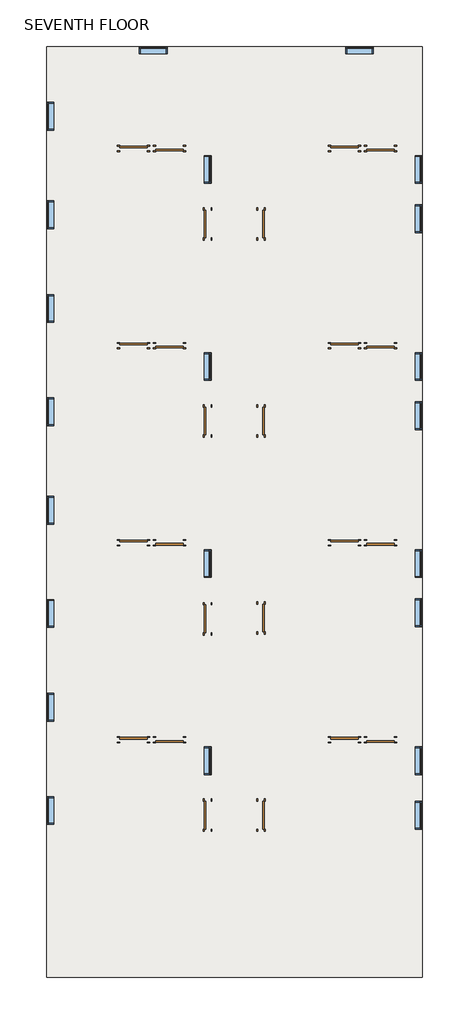
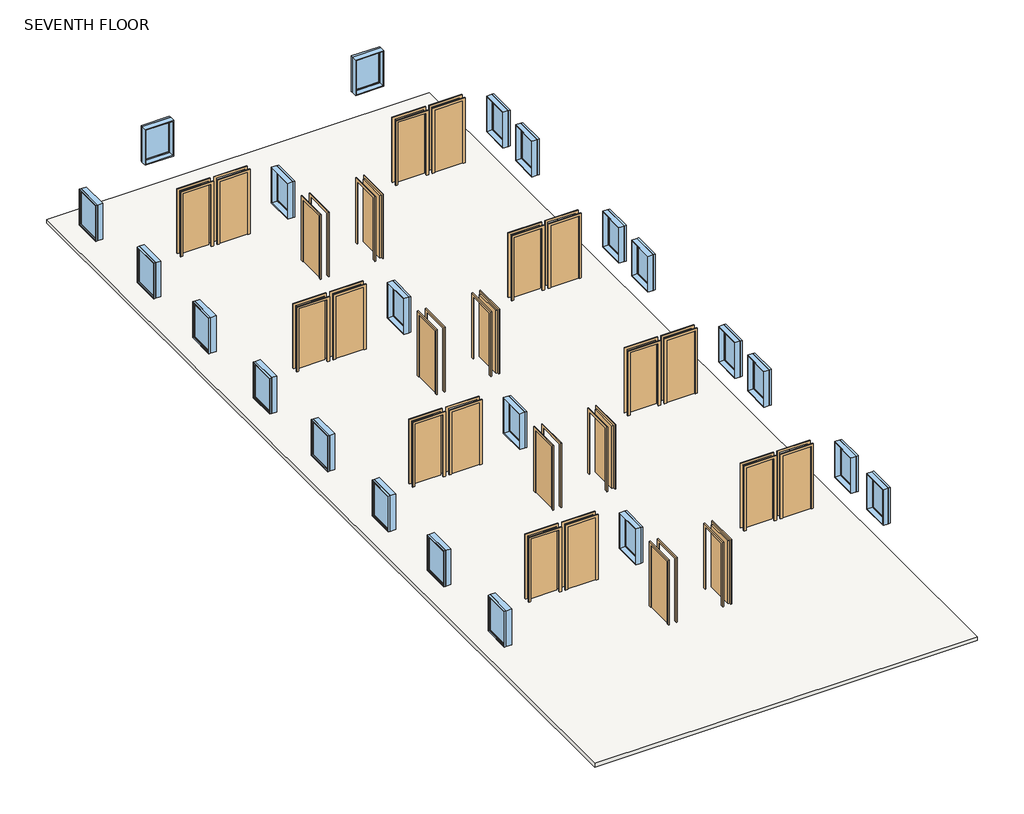
# One storey: 24 doors, 22 windows, 1 slab.
"""IFC4 building model written with IfcOpenShell, lengths in millimetres."""

from ifc_helpers import new_model, si_unit, frame, origin, place, context, project, spatial, polyline, outline, extrude, transform, mapped, element, save
from components import door_686f89d2, door_16372e1c, door_a90ba1ad, door_0ca8825f, window_c1f32544

model = new_model("IFC4")

# Units and contexts
model_context = context("Model", 3, world=origin())
ifc_project = project(units=[si_unit("LENGTHUNIT", "METRE", prefix="MILLI")], contexts=[model_context])

# Site, building, storey
site = spatial("IfcSite", under=ifc_project)
building = spatial("IfcBuilding", under=site)
storey = spatial("IfcBuildingStorey", under=building, Name="SEVENTH FLOOR", Elevation=22402.8)

# Doors
placement = place(None, origin())
door_shape = door_686f89d2(model_context)
element("IfcDoor", 1, ObjectType="Single-Flush : 36\" x 84\"", at=placement, inside=storey, context=model_context, shape_type="MappedRepresentation", body=[
    mapped(door_shape, transform((-9863.5902461, 11952.2710592, 22402.8), x_axis=(-1.0, 0.0, 0.0), y_axis=(0.0, -1.0, 0.0), z_axis=(0.0, 0.0, 1.0))),
])
element("IfcDoor", 2, ObjectType="Single-Flush : 36\" x 84\"", at=placement, inside=storey, context=model_context, shape_type="MappedRepresentation", body=[
    mapped(door_shape, transform((-9863.5902461, 5475.2710592, 22402.8), x_axis=(-1.0, 0.0, 0.0), y_axis=(0.0, -1.0, 0.0), z_axis=(0.0, 0.0, 1.0))),
])
element("IfcDoor", 3, ObjectType="Single-Flush : 36\" x 84\"", at=placement, inside=storey, context=model_context, shape_type="MappedRepresentation", body=[
    mapped(door_shape, transform((-9863.5902461, -1001.7289408, 22402.8), x_axis=(-1.0, 0.0, 0.0), y_axis=(0.0, -1.0, 0.0), z_axis=(0.0, 0.0, 1.0))),
])
element("IfcDoor", 4, ObjectType="Single-Flush : 36\" x 84\"", at=placement, inside=storey, context=model_context, shape_type="MappedRepresentation", body=[
    mapped(door_shape, transform((-9863.5902461, -7478.7289408, 22402.8), x_axis=(-1.0, 0.0, 0.0), y_axis=(0.0, -1.0, 0.0), z_axis=(0.0, 0.0, 1.0))),
])
element("IfcDoor", 5, ObjectType="Single-Flush : 36\" x 84\"", at=placement, inside=storey, context=model_context, shape_type="MappedRepresentation", body=[
    mapped(door_shape, transform((-2929.3902461, -7478.7289408, 22402.8), x_axis=(-1.0, 0.0, 0.0), y_axis=(0.0, -1.0, 0.0), z_axis=(0.0, 0.0, 1.0))),
])
element("IfcDoor", 6, ObjectType="Single-Flush : 36\" x 84\"", at=placement, inside=storey, context=model_context, shape_type="MappedRepresentation", body=[
    mapped(door_shape, transform((-2929.3902461, -1001.7289408, 22402.8), x_axis=(-1.0, 0.0, 0.0), y_axis=(0.0, -1.0, 0.0), z_axis=(0.0, 0.0, 1.0))),
])
element("IfcDoor", 7, ObjectType="Single-Flush : 36\" x 84\"", at=placement, inside=storey, context=model_context, shape_type="MappedRepresentation", body=[
    mapped(door_shape, transform((-2929.3902461, 5475.2710592, 22402.8), x_axis=(-1.0, 0.0, 0.0), y_axis=(0.0, -1.0, 0.0), z_axis=(0.0, 0.0, 1.0))),
])
element("IfcDoor", 8, ObjectType="Single-Flush : 36\" x 84\"", at=placement, inside=storey, context=model_context, shape_type="MappedRepresentation", body=[
    mapped(door_shape, transform((-2929.3902461, 11952.2710592, 22402.8), x_axis=(-1.0, 0.0, 0.0), y_axis=(0.0, -1.0, 0.0), z_axis=(0.0, 0.0, 1.0))),
])
door_2_shape = door_16372e1c(model_context)
element("IfcDoor", 9, ObjectType="Single-Flush : 36\" x 84\"", at=placement, inside=storey, context=model_context, shape_type="MappedRepresentation", body=[
    mapped(door_2_shape, transform((-8682.4902461, 11952.2710592, 22402.8), x_axis=(-1.0, 0.0, 0.0), y_axis=(0.0, -1.0, 0.0), z_axis=(0.0, 0.0, 1.0))),
])
element("IfcDoor", 10, ObjectType="Single-Flush : 36\" x 84\"", at=placement, inside=storey, context=model_context, shape_type="MappedRepresentation", body=[
    mapped(door_2_shape, transform((-8682.4902461, 5475.2710592, 22402.8), x_axis=(-1.0, 0.0, 0.0), y_axis=(0.0, -1.0, 0.0), z_axis=(0.0, 0.0, 1.0))),
])
element("IfcDoor", 11, ObjectType="Single-Flush : 36\" x 84\"", at=placement, inside=storey, context=model_context, shape_type="MappedRepresentation", body=[
    mapped(door_2_shape, transform((-8682.4902461, -1001.7289408, 22402.8), x_axis=(-1.0, 0.0, 0.0), y_axis=(0.0, -1.0, 0.0), z_axis=(0.0, 0.0, 1.0))),
])
element("IfcDoor", 12, ObjectType="Single-Flush : 36\" x 84\"", at=placement, inside=storey, context=model_context, shape_type="MappedRepresentation", body=[
    mapped(door_2_shape, transform((-8682.4902461, -7478.7289408, 22402.8), x_axis=(-1.0, 0.0, 0.0), y_axis=(0.0, -1.0, 0.0), z_axis=(0.0, 0.0, 1.0))),
])
element("IfcDoor", 13, ObjectType="Single-Flush : 36\" x 84\"", at=placement, inside=storey, context=model_context, shape_type="MappedRepresentation", body=[
    mapped(door_2_shape, transform((-1748.2902461, -7478.7289408, 22402.8), x_axis=(-1.0, 0.0, 0.0), y_axis=(0.0, -1.0, 0.0), z_axis=(0.0, 0.0, 1.0))),
])
element("IfcDoor", 14, ObjectType="Single-Flush : 36\" x 84\"", at=placement, inside=storey, context=model_context, shape_type="MappedRepresentation", body=[
    mapped(door_2_shape, transform((-1748.2902461, -1001.7289408, 22402.8), x_axis=(-1.0, 0.0, 0.0), y_axis=(0.0, -1.0, 0.0), z_axis=(0.0, 0.0, 1.0))),
])
element("IfcDoor", 15, ObjectType="Single-Flush : 36\" x 84\"", at=placement, inside=storey, context=model_context, shape_type="MappedRepresentation", body=[
    mapped(door_2_shape, transform((-1748.2902461, 5475.2710592, 22402.8), x_axis=(-1.0, 0.0, 0.0), y_axis=(0.0, -1.0, 0.0), z_axis=(0.0, 0.0, 1.0))),
])
element("IfcDoor", 16, ObjectType="Single-Flush : 36\" x 84\"", at=placement, inside=storey, context=model_context, shape_type="MappedRepresentation", body=[
    mapped(door_2_shape, transform((-1748.2902461, 11952.2710592, 22402.8), x_axis=(-1.0, 0.0, 0.0), y_axis=(0.0, -1.0, 0.0), z_axis=(0.0, 0.0, 1.0))),
])
door_3_shape = door_a90ba1ad(model_context)
element("IfcDoor", 17, ObjectType="Single-Flush : 36\" x 84\"", at=placement, inside=storey, context=model_context, shape_type="MappedRepresentation", body=[
    mapped(door_3_shape, transform((-7425.1902461, 9475.7710592, 22402.8), x_axis=(0.0, -1.0, 0.0), y_axis=(1.0, 0.0, 0.0), z_axis=(0.0, 0.0, 1.0))),
])
element("IfcDoor", 18, ObjectType="Single-Flush : 36\" x 84\"", at=placement, inside=storey, context=model_context, shape_type="MappedRepresentation", body=[
    mapped(door_3_shape, transform((-7425.1902461, 2998.7710592, 22402.8), x_axis=(0.0, -1.0, 0.0), y_axis=(1.0, 0.0, 0.0), z_axis=(0.0, 0.0, 1.0))),
])
element("IfcDoor", 19, ObjectType="Single-Flush : 36\" x 84\"", at=placement, inside=storey, context=model_context, shape_type="MappedRepresentation", body=[
    mapped(door_3_shape, transform((-7425.1902461, -3503.6289408, 22402.8), x_axis=(0.0, -1.0, 0.0), y_axis=(1.0, 0.0, 0.0), z_axis=(0.0, 0.0, 1.0))),
])
element("IfcDoor", 20, ObjectType="Single-Flush : 36\" x 84\"", at=placement, inside=storey, context=model_context, shape_type="MappedRepresentation", body=[
    mapped(door_3_shape, transform((-7425.1902461, -9955.2289408, 22402.8), x_axis=(0.0, -1.0, 0.0), y_axis=(1.0, 0.0, 0.0), z_axis=(0.0, 0.0, 1.0))),
])
door_4_shape = door_0ca8825f(model_context)
element("IfcDoor", 21, ObjectType="Single-Flush : 36\" x 84\"", at=placement, inside=storey, context=model_context, shape_type="MappedRepresentation", body=[
    mapped(door_4_shape, transform((-5672.5902461, 9475.7710592, 22402.8), x_axis=(0.0, -1.0, 0.0), y_axis=(1.0, 0.0, 0.0), z_axis=(0.0, 0.0, 1.0))),
])
element("IfcDoor", 22, ObjectType="Single-Flush : 36\" x 84\"", at=placement, inside=storey, context=model_context, shape_type="MappedRepresentation", body=[
    mapped(door_4_shape, transform((-5672.5902461, 2998.7710592, 22402.8), x_axis=(0.0, -1.0, 0.0), y_axis=(1.0, 0.0, 0.0), z_axis=(0.0, 0.0, 1.0))),
])
element("IfcDoor", 23, ObjectType="Single-Flush : 36\" x 84\"", at=placement, inside=storey, context=model_context, shape_type="MappedRepresentation", body=[
    mapped(door_4_shape, transform((-5672.5902461, -3478.2289408, 22402.8), x_axis=(0.0, -1.0, 0.0), y_axis=(1.0, 0.0, 0.0), z_axis=(0.0, 0.0, 1.0))),
])
element("IfcDoor", 24, ObjectType="Single-Flush : 36\" x 84\"", at=placement, inside=storey, context=model_context, shape_type="MappedRepresentation", body=[
    mapped(door_4_shape, transform((-5672.5902461, -9955.2289408, 22402.8), x_axis=(0.0, -1.0, 0.0), y_axis=(1.0, 0.0, 0.0), z_axis=(0.0, 0.0, 1.0))),
])

# Slab
element("IfcSlab", 25, ObjectType="Generic - 12\"", at=placement, inside=storey, context=model_context, shape_type="SweptSolid", body=[
    extrude(outline(polyline([(-376.6902461, 15305.0710592), (-376.6902461, -15289.2289408), (-12721.0902461, -15289.2289408), (-12721.0902461, 15305.0710592), (-376.6902461, 15305.0710592)])), frame((0.0, 0.0, 22275.8), z_axis=(0.0, 0.0, 1.0), x_axis=(1.0, 0.0, 0.0)), (0.0, 0.0, 1.0), 127.0),
])

# Windows
window_shape = window_c1f32544(model_context)
element("IfcWindow", 26, ObjectType="Fixed : 36\" x 48\"", at=placement, inside=storey, context=model_context, shape_type="MappedRepresentation", body=[
    mapped(window_shape, transform((-9177.7902461, 15190.7710592, 22402.8), x_axis=(1.0, 0.0, 0.0), y_axis=(0.0, 1.0, 0.0), z_axis=(0.0, 0.0, 1.0))),
])
element("IfcWindow", 27, ObjectType="Fixed : 36\" x 48\"", at=placement, inside=storey, context=model_context, shape_type="MappedRepresentation", body=[
    mapped(window_shape, transform((-2395.9902461, 15190.7710592, 22402.8), x_axis=(1.0, 0.0, 0.0), y_axis=(0.0, 1.0, 0.0), z_axis=(0.0, 0.0, 1.0))),
])
element("IfcWindow", 28, ObjectType="Fixed : 36\" x 48\"", at=placement, inside=storey, context=model_context, shape_type="MappedRepresentation", body=[
    mapped(window_shape, transform((-490.9902461, 11228.3710592, 22402.8), x_axis=(0.0, -1.0, 0.0), y_axis=(1.0, 0.0, 0.0), z_axis=(0.0, 0.0, 1.0))),
])
element("IfcWindow", 29, ObjectType="Fixed : 36\" x 48\"", at=placement, inside=storey, context=model_context, shape_type="MappedRepresentation", body=[
    mapped(window_shape, transform((-490.9902461, 9609.1210592, 22402.8), x_axis=(0.0, -1.0, 0.0), y_axis=(1.0, 0.0, 0.0), z_axis=(0.0, 0.0, 1.0))),
])
element("IfcWindow", 30, ObjectType="Fixed : 36\" x 48\"", at=placement, inside=storey, context=model_context, shape_type="MappedRepresentation", body=[
    mapped(window_shape, transform((-490.9902461, 4751.3710592, 22402.8), x_axis=(0.0, -1.0, 0.0), y_axis=(1.0, 0.0, 0.0), z_axis=(0.0, 0.0, 1.0))),
])
element("IfcWindow", 31, ObjectType="Fixed : 36\" x 48\"", at=placement, inside=storey, context=model_context, shape_type="MappedRepresentation", body=[
    mapped(window_shape, transform((-490.9902461, 3132.1210592, 22402.8), x_axis=(0.0, -1.0, 0.0), y_axis=(1.0, 0.0, 0.0), z_axis=(0.0, 0.0, 1.0))),
])
element("IfcWindow", 32, ObjectType="Fixed : 36\" x 48\"", at=placement, inside=storey, context=model_context, shape_type="MappedRepresentation", body=[
    mapped(window_shape, transform((-490.9902461, -1725.6289408, 22402.8), x_axis=(0.0, -1.0, 0.0), y_axis=(1.0, 0.0, 0.0), z_axis=(0.0, 0.0, 1.0))),
])
element("IfcWindow", 33, ObjectType="Fixed : 36\" x 48\"", at=placement, inside=storey, context=model_context, shape_type="MappedRepresentation", body=[
    mapped(window_shape, transform((-490.9902461, -3344.8789408, 22402.8), x_axis=(0.0, -1.0, 0.0), y_axis=(1.0, 0.0, 0.0), z_axis=(0.0, 0.0, 1.0))),
])
element("IfcWindow", 34, ObjectType="Fixed : 36\" x 48\"", at=placement, inside=storey, context=model_context, shape_type="MappedRepresentation", body=[
    mapped(window_shape, transform((-490.9902461, -8202.6289408, 22402.8), x_axis=(0.0, -1.0, 0.0), y_axis=(1.0, 0.0, 0.0), z_axis=(0.0, 0.0, 1.0))),
])
element("IfcWindow", 35, ObjectType="Fixed : 36\" x 48\"", at=placement, inside=storey, context=model_context, shape_type="MappedRepresentation", body=[
    mapped(window_shape, transform((-490.9902461, -9993.3289408, 22402.8), x_axis=(0.0, -1.0, 0.0), y_axis=(1.0, 0.0, 0.0), z_axis=(0.0, 0.0, 1.0))),
])
element("IfcWindow", 36, ObjectType="Fixed : 36\" x 48\"", at=placement, inside=storey, context=model_context, shape_type="MappedRepresentation", body=[
    mapped(window_shape, transform((-12606.7902461, -9764.7289408, 22402.8), x_axis=(0.0, 1.0, 0.0), y_axis=(-1.0, 0.0, 0.0), z_axis=(0.0, 0.0, 1.0))),
])
element("IfcWindow", 37, ObjectType="Fixed : 36\" x 48\"", at=placement, inside=storey, context=model_context, shape_type="MappedRepresentation", body=[
    mapped(window_shape, transform((-12606.7902461, -6373.8289408, 22402.8), x_axis=(0.0, 1.0, 0.0), y_axis=(-1.0, 0.0, 0.0), z_axis=(0.0, 0.0, 1.0))),
])
element("IfcWindow", 38, ObjectType="Fixed : 36\" x 48\"", at=placement, inside=storey, context=model_context, shape_type="MappedRepresentation", body=[
    mapped(window_shape, transform((-12606.7902461, -3287.7289408, 22402.8), x_axis=(0.0, 1.0, 0.0), y_axis=(-1.0, 0.0, 0.0), z_axis=(0.0, 0.0, 1.0))),
])
element("IfcWindow", 39, ObjectType="Fixed : 36\" x 48\"", at=placement, inside=storey, context=model_context, shape_type="MappedRepresentation", body=[
    mapped(window_shape, transform((-12606.7902461, 103.1710592, 22402.8), x_axis=(0.0, 1.0, 0.0), y_axis=(-1.0, 0.0, 0.0), z_axis=(0.0, 0.0, 1.0))),
])
element("IfcWindow", 40, ObjectType="Fixed : 36\" x 48\"", at=placement, inside=storey, context=model_context, shape_type="MappedRepresentation", body=[
    mapped(window_shape, transform((-12606.7902461, 3341.6710592, 22402.8), x_axis=(0.0, 1.0, 0.0), y_axis=(-1.0, 0.0, 0.0), z_axis=(0.0, 0.0, 1.0))),
])
element("IfcWindow", 41, ObjectType="Fixed : 36\" x 48\"", at=placement, inside=storey, context=model_context, shape_type="MappedRepresentation", body=[
    mapped(window_shape, transform((-12606.7902461, 6732.5710592, 22402.8), x_axis=(0.0, 1.0, 0.0), y_axis=(-1.0, 0.0, 0.0), z_axis=(0.0, 0.0, 1.0))),
])
element("IfcWindow", 42, ObjectType="Fixed : 36\" x 48\"", at=placement, inside=storey, context=model_context, shape_type="MappedRepresentation", body=[
    mapped(window_shape, transform((-12606.7902461, 9818.6710592, 22402.8), x_axis=(0.0, 1.0, 0.0), y_axis=(-1.0, 0.0, 0.0), z_axis=(0.0, 0.0, 1.0))),
])
element("IfcWindow", 43, ObjectType="Fixed : 36\" x 48\"", at=placement, inside=storey, context=model_context, shape_type="MappedRepresentation", body=[
    mapped(window_shape, transform((-12606.7902461, 13057.1710592, 22402.8), x_axis=(0.0, 1.0, 0.0), y_axis=(-1.0, 0.0, 0.0), z_axis=(0.0, 0.0, 1.0))),
])
element("IfcWindow", 44, ObjectType="Fixed : 36\" x 48\"", at=placement, inside=storey, context=model_context, shape_type="MappedRepresentation", body=[
    mapped(window_shape, transform((-7425.1902461, 4751.3710592, 22402.8), x_axis=(0.0, -1.0, 0.0), y_axis=(1.0, 0.0, 0.0), z_axis=(0.0, 0.0, 1.0))),
])
element("IfcWindow", 45, ObjectType="Fixed : 36\" x 48\"", at=placement, inside=storey, context=model_context, shape_type="MappedRepresentation", body=[
    mapped(window_shape, transform((-7425.1902461, 11228.3710592, 22402.8), x_axis=(0.0, -1.0, 0.0), y_axis=(1.0, 0.0, 0.0), z_axis=(0.0, 0.0, 1.0))),
])
element("IfcWindow", 46, ObjectType="Fixed : 36\" x 48\"", at=placement, inside=storey, context=model_context, shape_type="MappedRepresentation", body=[
    mapped(window_shape, transform((-7425.1902461, -1725.6289408, 22402.8), x_axis=(0.0, -1.0, 0.0), y_axis=(1.0, 0.0, 0.0), z_axis=(0.0, 0.0, 1.0))),
])
element("IfcWindow", 47, ObjectType="Fixed : 36\" x 48\"", at=placement, inside=storey, context=model_context, shape_type="MappedRepresentation", body=[
    mapped(window_shape, transform((-7425.1902461, -8202.6289408, 22402.8), x_axis=(0.0, -1.0, 0.0), y_axis=(1.0, 0.0, 0.0), z_axis=(0.0, 0.0, 1.0))),
])

save(model, "model.ifc")

# Revit data of these elements
# Type "Single-Flush : 36\" x 84\""
#   Type Mark = "1"
#   Construction Type Id = "MDOOR"
#   Assembly Code = "C1020"
#   Analytic Construction = "Metal"
#   Thickness = 0' - 2"
#   Heat Transfer Coefficient (U) = 0.651978 BTU/(h·ft²·°F)
#   Height = 7' - 0"
#   Trim Projection Ext = 0' - 1"
#   Trim Projection Int = 0' - 1"
#   Trim Width = 0' - 3"
#   Width = 3' - 0"
#   Define Thermal Properties by = 1
#   Door Material = Door - Panel
#   Frame Material = Door - Frame
#   Visual Light Transmittance = 0
#   Solar Heat Gain Coefficient = 0
#   Function = (empty or 0)
#   Wall Closure = (empty or 0)
# Type "Generic - 12\""
#   Assembly Code = "B1010"
#   Function = 0
#   Layers, outside or top first: 0' - 5" no material (function 1)
# Type "Fixed : 36\" x 48\""
#   Type Mark = "1"
#   Construction Type Id = "GSP4R"
#   Assembly Code = "B2020100"
#   Analytic Construction = "1/8 in Pilkington single glazing"
#   Visual Light Transmittance = 0.9
#   Solar Heat Gain Coefficient = 0.78
#   Heat Transfer Coefficient (U) = 0.6496 BTU/(h·ft²·°F)
#   Height = 4' - 0"
#   Default Sill Height = 3' - 0"
#   Width = 3' - 0"
#   Window Inset = 0' - 0 3/4"
#   Define Thermal Properties by = 1
#   Glass Pane Material = Glass
#   Sash Material = Sash
#   Wall Closure = (empty or 0)
# Elements 1, 2, 3, 4, 5, 6, 7, 8, 9, 10, 11, 12, 13, 14, 15, 16, 17, 18, 19, 20, 21, 22, 23, 24 (IfcDoor, "Single-Flush : 36\" x 84\"")
#   Phase Created = New Construction
#   Materials on its faces: "Door - Frame", "Door - Panel"
# Element 25 (IfcSlab, "Generic - 12\"")
#   Height Offset From Level = 0' - 0"
#   Phase Created = New Construction
#   Materials on its faces: "Default Floor"
# Element 26 (IfcWindow, "Fixed : 36\" x 48\"")
#   Mark = "161"
#   Phase Created = New Construction
#   Materials on its faces: "Sash", "Glass"
# Element 27 (IfcWindow, "Fixed : 36\" x 48\"")
#   Mark = "162"
#   Phase Created = New Construction
#   Materials on its faces: "Sash", "Glass"
# Element 28 (IfcWindow, "Fixed : 36\" x 48\"")
#   Mark = "163"
#   Phase Created = New Construction
#   Materials on its faces: "Sash", "Glass"
# Element 29 (IfcWindow, "Fixed : 36\" x 48\"")
#   Mark = "164"
#   Phase Created = New Construction
#   Materials on its faces: "Sash", "Glass"
# Element 30 (IfcWindow, "Fixed : 36\" x 48\"")
#   Mark = "165"
#   Phase Created = New Construction
#   Materials on its faces: "Sash", "Glass"
# Element 31 (IfcWindow, "Fixed : 36\" x 48\"")
#   Mark = "166"
#   Phase Created = New Construction
#   Materials on its faces: "Sash", "Glass"
# Element 32 (IfcWindow, "Fixed : 36\" x 48\"")
#   Mark = "167"
#   Phase Created = New Construction
#   Materials on its faces: "Sash", "Glass"
# Element 33 (IfcWindow, "Fixed : 36\" x 48\"")
#   Mark = "168"
#   Phase Created = New Construction
#   Materials on its faces: "Sash", "Glass"
# Element 34 (IfcWindow, "Fixed : 36\" x 48\"")
#   Mark = "169"
#   Phase Created = New Construction
#   Materials on its faces: "Sash", "Glass"
# Element 35 (IfcWindow, "Fixed : 36\" x 48\"")
#   Mark = "170"
#   Phase Created = New Construction
#   Materials on its faces: "Sash", "Glass"
# Element 36 (IfcWindow, "Fixed : 36\" x 48\"")
#   Mark = "171"
#   Phase Created = New Construction
#   Materials on its faces: "Sash", "Glass"
# Element 37 (IfcWindow, "Fixed : 36\" x 48\"")
#   Mark = "172"
#   Phase Created = New Construction
#   Materials on its faces: "Sash", "Glass"
# Element 38 (IfcWindow, "Fixed : 36\" x 48\"")
#   Mark = "173"
#   Phase Created = New Construction
#   Materials on its faces: "Sash", "Glass"
# Element 39 (IfcWindow, "Fixed : 36\" x 48\"")
#   Mark = "174"
#   Phase Created = New Construction
#   Materials on its faces: "Sash", "Glass"
# Element 40 (IfcWindow, "Fixed : 36\" x 48\"")
#   Mark = "175"
#   Phase Created = New Construction
#   Materials on its faces: "Sash", "Glass"
# Element 41 (IfcWindow, "Fixed : 36\" x 48\"")
#   Mark = "176"
#   Phase Created = New Construction
#   Materials on its faces: "Sash", "Glass"
# Element 42 (IfcWindow, "Fixed : 36\" x 48\"")
#   Mark = "177"
#   Phase Created = New Construction
#   Materials on its faces: "Sash", "Glass"
# Element 43 (IfcWindow, "Fixed : 36\" x 48\"")
#   Mark = "178"
#   Phase Created = New Construction
#   Materials on its faces: "Sash", "Glass"
# Element 44 (IfcWindow, "Fixed : 36\" x 48\"")
#   Mark = "179"
#   Phase Created = New Construction
#   Materials on its faces: "Sash", "Glass"
# Element 45 (IfcWindow, "Fixed : 36\" x 48\"")
#   Mark = "180"
#   Phase Created = New Construction
#   Materials on its faces: "Sash", "Glass"
# Element 46 (IfcWindow, "Fixed : 36\" x 48\"")
#   Mark = "181"
#   Phase Created = New Construction
#   Materials on its faces: "Sash", "Glass"
# Element 47 (IfcWindow, "Fixed : 36\" x 48\"")
#   Mark = "182"
#   Phase Created = New Construction
#   Materials on its faces: "Sash", "Glass"
# Materials
#   "Door - Panel": class "Wood", colour RGB 210 159 95, transparency 0
#   "Door - Frame": colour RGB 118 70 51, transparency 0
#   "Glass": class "Glass", colour RGB 0 128 192, transparency 0.75, Description = "Soda Lime Glass", Cost = 0
#   "Sash": class "Wood", colour RGB 224 178 126, transparency 0
#   "Default Floor": colour RGB 128 128 128, transparency 0
